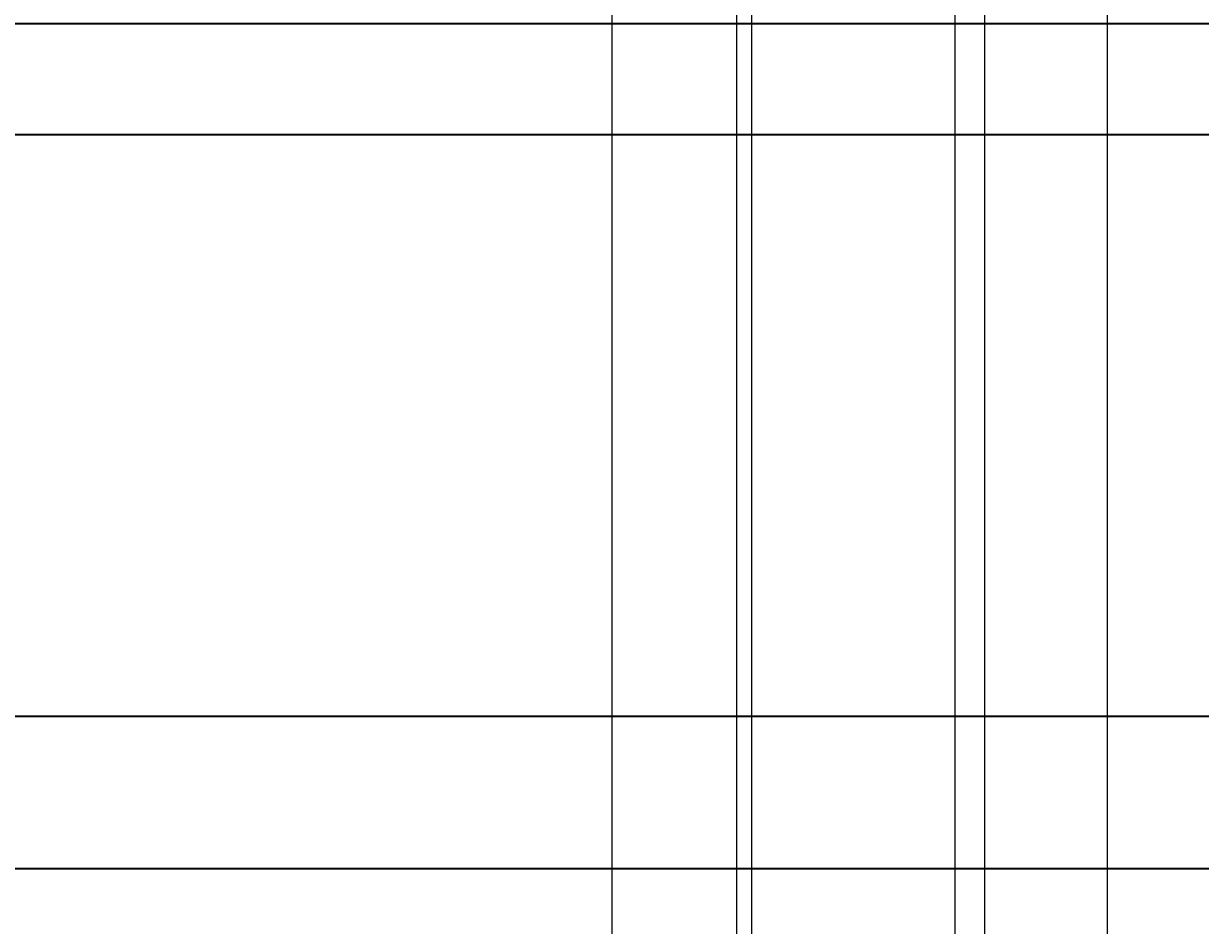
# Model space of a CAD drawing. Units: inches. Extents: x -6 to 289, y -8 to 323.
# Tile 89 of 107: x 150 to 173, y 276 to 294. Entities that reach past the tile are written whole.
import ezdxf

# ---------------------------------------------------------------- set-up
doc = ezdxf.new("R2010")
doc.units = ezdxf.units.IN
doc.header["$MEASUREMENT"] = 0
doc.layers.add('A-ANNO-DIMS', color=2, linetype='Continuous', lineweight=18)
doc.layers.add('A-ELEV', color=7, linetype='Continuous', lineweight=35)
doc.styles.get("Standard").update_dxf_attribs({"font": 'arial.ttf'})
doc.dimstyles.get("Standard").update_dxf_attribs({"dimtxt": 0.18, "dimasz": 0.18, "dimexe": 0.18, "dimexo": 0.0625, "dimgap": 0.09, "dimtad": 0, "dimtih": 1, "dimtoh": 1, "dimdec": 4, "dimzin": 0, "dimdsep": 46, "dimtxsty": 'Standard', "dimcen": 0.09, "dimadec": 0, "dimazin": 0, "dimtfac": 1, "dimtdec": 4, "dimtofl": 0, "dimtmove": 0, "dimatfit": 3, "dimfxl": 1, "dimtolj": 1, "dimtzin": 0, "dimarcsym": 0})

# ---------------------------------------------------------------- blocks, each defined once
blk = doc.blocks.new('*D11')
at = {"layer": 'A-ANNO-DIMS', "color": 0, "lineweight": -2, "transparency": 16777216}
for p, q in [((126.883, 226.717), (126.883, 322.969)), ((168.883, 226.717), (168.883, 322.969)), ((127.063, 322.789), (147.662, 322.789)), ((168.703, 322.789), (148.105, 322.789))]:
    blk.add_line(p, q, dxfattribs=at)
at = {"layer": 'A-ANNO-DIMS', "color": 0, "transparency": 16777216}
for points in [[(127.063, 322.819), (127.063, 322.759), (126.883, 322.789)], [(168.703, 322.819), (168.703, 322.759), (168.883, 322.789)]]:
    blk.add_solid(points, dxfattribs=at)
at = {"layer": 'Defpoints', "color": 0, "transparency": 16777216}
for p in [(168.883, 322.789), (126.883, 226.654), (168.883, 226.654)]:
    blk.add_point(p, dxfattribs=at)
at = {"layer": 'A-ANNO-DIMS', "color": 0, "transparency": 16777216, "insert": (147.883, 322.789), "char_height": 0.18, "attachment_point": 5}
blk.add_mtext('\\A1;42', dxfattribs=at)
blk = doc.blocks.new('*D12')
at = {"layer": 'A-ANNO-DIMS', "color": 0, "lineweight": -2, "transparency": 16777216}
for p, q in [((168.883, 226.717), (168.883, 322.969)), ((188.292, 226.951), (188.292, 322.969)), ((169.063, 322.789), (178.22, 322.789)), ((188.112, 322.789), (178.955, 322.789))]:
    blk.add_line(p, q, dxfattribs=at)
at = {"layer": 'A-ANNO-DIMS', "color": 0, "transparency": 16777216}
for points in [[(169.063, 322.819), (169.063, 322.759), (168.883, 322.789)], [(188.112, 322.819), (188.112, 322.759), (188.292, 322.789)]]:
    blk.add_solid(points, dxfattribs=at)
at = {"layer": 'Defpoints', "color": 0, "transparency": 16777216}
for p in [(188.292, 322.789), (188.292, 226.889), (168.883, 226.654)]:
    blk.add_point(p, dxfattribs=at)
at = {"layer": 'A-ANNO-DIMS', "color": 0, "transparency": 16777216, "insert": (178.588, 322.789), "char_height": 0.18, "attachment_point": 5}
blk.add_mtext('\\A1;19.41', dxfattribs=at)
blk = doc.blocks.new('*D27')
at = {"layer": 'A-ANNO-DIMS', "color": 0, "lineweight": -2, "transparency": 16777216}
for p, q in [((19.226, 307.289), (288.653, 307.289)), ((288.473, 307.109), (288.473, 277.471)), ((288.473, 247.469), (288.473, 277.107)), ((247.226, 247.289), (288.653, 247.289))]:
    blk.add_line(p, q, dxfattribs=at)
at = {"layer": 'A-ANNO-DIMS', "color": 0, "transparency": 16777216}
for points in [[(288.443, 307.109), (288.503, 307.109), (288.473, 307.289)], [(288.443, 247.469), (288.503, 247.469), (288.473, 247.289)]]:
    blk.add_solid(points, dxfattribs=at)
at = {"layer": 'Defpoints', "color": 0, "transparency": 16777216}
for p in [(19.164, 307.289), (288.473, 307.289), (247.164, 247.289)]:
    blk.add_point(p, dxfattribs=at)
at = {"layer": 'A-ANNO-DIMS', "color": 0, "transparency": 16777216, "insert": (288.473, 277.289), "char_height": 0.18, "attachment_point": 5}
blk.add_mtext('\\A1;60', dxfattribs=at)
blk = doc.blocks.new('*D76')
at = {"layer": 'A-ANNO-DIMS', "color": 0, "lineweight": -2, "transparency": 16777216}
for p, q in [((142.296, 51.148), (142.296, 322.969)), ((164.296, 51.148), (164.296, 322.969)), ((142.476, 322.789), (153.076, 322.789)), ((164.116, 322.789), (153.516, 322.789))]:
    blk.add_line(p, q, dxfattribs=at)
at = {"layer": 'A-ANNO-DIMS', "color": 0, "transparency": 16777216}
for points in [[(142.476, 322.819), (142.476, 322.759), (142.296, 322.789)], [(164.116, 322.819), (164.116, 322.759), (164.296, 322.789)]]:
    blk.add_solid(points, dxfattribs=at)
at = {"layer": 'Defpoints', "color": 0, "transparency": 16777216}
for p in [(164.296, 322.789), (142.296, 51.085), (164.296, 51.085)]:
    blk.add_point(p, dxfattribs=at)
at = {"layer": 'A-ANNO-DIMS', "color": 0, "transparency": 16777216, "insert": (153.296, 322.789), "char_height": 0.18, "attachment_point": 5}
blk.add_mtext('\\A1;22', dxfattribs=at)
blk = doc.blocks.new('*D77')
at = {"layer": 'A-ANNO-DIMS', "color": 0, "lineweight": -2, "transparency": 16777216}
for p, q in [((164.296, 51.148), (164.296, 322.969)), ((168.296, 51.148), (168.296, 322.969)), ((164.476, 322.789), (166.144, 322.789)), ((168.116, 322.789), (166.448, 322.789))]:
    blk.add_line(p, q, dxfattribs=at)
at = {"layer": 'A-ANNO-DIMS', "color": 0, "transparency": 16777216}
for points in [[(164.476, 322.819), (164.476, 322.759), (164.296, 322.789)], [(168.116, 322.819), (168.116, 322.759), (168.296, 322.789)]]:
    blk.add_solid(points, dxfattribs=at)
at = {"layer": 'Defpoints', "color": 0, "transparency": 16777216}
for p in [(168.296, 322.789), (164.296, 51.085), (168.296, 51.085)]:
    blk.add_point(p, dxfattribs=at)
at = {"layer": 'A-ANNO-DIMS', "color": 0, "transparency": 16777216, "insert": (166.296, 322.789), "char_height": 0.18, "attachment_point": 5}
blk.add_mtext('\\A1;4', dxfattribs=at)
blk = doc.blocks.new('*D78')
at = {"layer": 'A-ANNO-DIMS', "color": 0, "lineweight": -2, "transparency": 16777216}
for p, q in [((168.296, 51.148), (168.296, 322.969)), ((171.296, 51.148), (171.296, 322.969)), ((168.476, 322.789), (169.647, 322.789)), ((171.116, 322.789), (169.945, 322.789))]:
    blk.add_line(p, q, dxfattribs=at)
at = {"layer": 'A-ANNO-DIMS', "color": 0, "transparency": 16777216}
for points in [[(168.476, 322.819), (168.476, 322.759), (168.296, 322.789)], [(171.116, 322.819), (171.116, 322.759), (171.296, 322.789)]]:
    blk.add_solid(points, dxfattribs=at)
at = {"layer": 'Defpoints', "color": 0, "transparency": 16777216}
for p in [(171.296, 322.789), (168.296, 51.085), (171.296, 51.085)]:
    blk.add_point(p, dxfattribs=at)
at = {"layer": 'A-ANNO-DIMS', "color": 0, "transparency": 16777216, "insert": (169.796, 322.789), "char_height": 0.18, "attachment_point": 5}
blk.add_mtext('\\A1;3', dxfattribs=at)
blk = doc.blocks.new('*D79')
at = {"layer": 'A-ANNO-DIMS', "color": 0, "lineweight": -2, "transparency": 16777216}
for p, q in [((171.296, 118.033), (171.296, 322.969)), ((188.292, 116.842), (188.292, 322.969)), ((171.476, 322.789), (179.339, 322.789)), ((188.112, 322.789), (180.249, 322.789))]:
    blk.add_line(p, q, dxfattribs=at)
at = {"layer": 'A-ANNO-DIMS', "color": 0, "transparency": 16777216}
for points in [[(171.476, 322.819), (171.476, 322.759), (171.296, 322.789)], [(188.112, 322.819), (188.112, 322.759), (188.292, 322.789)]]:
    blk.add_solid(points, dxfattribs=at)
at = {"layer": 'Defpoints', "color": 0, "transparency": 16777216}
for p in [(188.292, 322.789), (171.296, 117.971), (188.292, 116.779)]:
    blk.add_point(p, dxfattribs=at)
at = {"layer": 'A-ANNO-DIMS', "color": 0, "transparency": 16777216, "insert": (179.794, 322.789), "char_height": 0.18, "attachment_point": 5}
blk.add_mtext('\\A1;16.996', dxfattribs=at)
blk = doc.blocks.new('*D94')
at = {"layer": 'A-ANNO-DIMS', "color": 0, "lineweight": -2, "transparency": 16777216}
for p, q in [((118.164, 159.411), (118.164, 322.969)), ((161.552, 159.411), (161.552, 322.969)), ((118.344, 322.789), (139.46, 322.789)), ((161.372, 322.789), (140.256, 322.789))]:
    blk.add_line(p, q, dxfattribs=at)
at = {"layer": 'A-ANNO-DIMS', "color": 0, "transparency": 16777216}
for points in [[(118.344, 322.819), (118.344, 322.759), (118.164, 322.789)], [(161.372, 322.819), (161.372, 322.759), (161.552, 322.789)]]:
    blk.add_solid(points, dxfattribs=at)
at = {"layer": 'Defpoints', "color": 0, "transparency": 16777216}
for p in [(161.552, 322.789), (118.164, 159.348), (161.552, 159.348)]:
    blk.add_point(p, dxfattribs=at)
at = {"layer": 'A-ANNO-DIMS', "color": 0, "transparency": 16777216, "insert": (139.858, 322.789), "char_height": 0.18, "attachment_point": 5}
blk.add_mtext('\\A1;43.39', dxfattribs=at)
blk = doc.blocks.new('*D95')
at = {"layer": 'A-ANNO-DIMS', "color": 0, "lineweight": -2, "transparency": 16777216}
for p, q in [((161.552, 159.411), (161.552, 322.969)), ((164.004, 159.411), (164.004, 322.969)), ((161.732, 322.789), (162.452, 322.789)), ((163.824, 322.789), (163.104, 322.789))]:
    blk.add_line(p, q, dxfattribs=at)
at = {"layer": 'A-ANNO-DIMS', "color": 0, "transparency": 16777216}
for points in [[(161.732, 322.819), (161.732, 322.759), (161.552, 322.789)], [(163.824, 322.819), (163.824, 322.759), (164.004, 322.789)]]:
    blk.add_solid(points, dxfattribs=at)
at = {"layer": 'Defpoints', "color": 0, "transparency": 16777216}
for p in [(164.004, 322.789), (161.552, 159.348), (164.004, 159.348)]:
    blk.add_point(p, dxfattribs=at)
at = {"layer": 'A-ANNO-DIMS', "color": 0, "transparency": 16777216, "insert": (162.778, 322.789), "char_height": 0.18, "attachment_point": 5}
blk.add_mtext('\\A1;2.45', dxfattribs=at)
blk = doc.blocks.new('*D96')
at = {"layer": 'A-ANNO-DIMS', "color": 0, "lineweight": -2, "transparency": 16777216}
for p, q in [((164.004, 159.411), (164.004, 322.969)), ((200.616, 159.411), (200.616, 322.969)), ((164.184, 322.789), (181.934, 322.789)), ((200.436, 322.789), (182.686, 322.789))]:
    blk.add_line(p, q, dxfattribs=at)
at = {"layer": 'A-ANNO-DIMS', "color": 0, "transparency": 16777216}
for points in [[(164.184, 322.819), (164.184, 322.759), (164.004, 322.789)], [(200.436, 322.819), (200.436, 322.759), (200.616, 322.789)]]:
    blk.add_solid(points, dxfattribs=at)
at = {"layer": 'Defpoints', "color": 0, "transparency": 16777216}
for p in [(200.616, 322.789), (164.004, 159.348), (200.616, 159.348)]:
    blk.add_point(p, dxfattribs=at)
at = {"layer": 'A-ANNO-DIMS', "color": 0, "transparency": 16777216, "insert": (182.31, 322.789), "char_height": 0.18, "attachment_point": 5}
blk.add_mtext('\\A1;36.61', dxfattribs=at)
blk = doc.blocks.new('*D107')
at = {"layer": 'A-ANNO-DIMS', "color": 0, "lineweight": -2, "transparency": 16777216}
for p, q in [((118.164, 293.728), (118.164, 322.969)), ((186.984, 291.541), (186.984, 322.969)), ((118.344, 322.789), (152.18, 322.789)), ((186.804, 322.789), (152.967, 322.789))]:
    blk.add_line(p, q, dxfattribs=at)
at = {"layer": 'A-ANNO-DIMS', "color": 0, "transparency": 16777216}
for points in [[(118.344, 322.819), (118.344, 322.759), (118.164, 322.789)], [(186.804, 322.819), (186.804, 322.759), (186.984, 322.789)]]:
    blk.add_solid(points, dxfattribs=at)
at = {"layer": 'Defpoints', "color": 0, "transparency": 16777216}
for p in [(186.984, 322.789), (118.164, 293.666), (186.984, 291.478)]:
    blk.add_point(p, dxfattribs=at)
at = {"layer": 'A-ANNO-DIMS', "color": 0, "transparency": 16777216, "insert": (152.574, 322.789), "char_height": 0.18, "attachment_point": 5}
blk.add_mtext('\\A1;68.82', dxfattribs=at)

msp = doc.modelspace()

# ---------------------------------------------------------------- linework, layer by layer
at = {"layer": 'A-ELEV'}
for points in [[(115.1638, 307.2888), (115.1638, 277.0427), (259.1638, 277.0427), (259.1638, 259.2888)], [(118.1638, 307.2888), (118.1638, 280.0427), (262.1638, 280.0427), (262.1638, 259.2888)], [(255.8036, 291.4781), (118.1638, 291.4781), (118.1638, 293.6657), (255.8036, 293.6657)]]:
    msp.add_lwpolyline(points, dxfattribs=at)

# ---------------------------------------------------------------- dimensions: what is measured, and where the dimension line sits
at = {"layer": 'A-ANNO-DIMS'}
for base, p1, p2, override, picture, middle in [((161.5522, 322.7888), (118.1638, 159.3484), (161.5522, 159.3484), {"dimdec": 2, "dimlfac": 1, "dimrnd": 0, "dimzin": 0, "dimdsep": 46, "dimlunit": 2}, '*D94', (139.858, 322.7888)), ((186.9837, 322.7888), (118.1638, 293.6657), (186.9837, 291.4781), {"dimdec": 2, "dimlfac": 1, "dimrnd": 0, "dimzin": 0, "dimdsep": 46, "dimlunit": 2}, '*D107', (152.5737, 322.7888)), ((168.8835, 322.7888), (126.8835, 226.654), (168.8835, 226.654), {"dimdec": 0, "dimlfac": 1, "dimrnd": 0, "dimzin": 0, "dimdsep": 46, "dimlunit": 2}, '*D11', (147.8835, 322.7888)), ((164.296, 322.7888), (142.296, 51.0851), (164.296, 51.0851), {"dimdec": 0, "dimlfac": 1, "dimrnd": 0, "dimzin": 0, "dimdsep": 46, "dimlunit": 2}, '*D76', (153.296, 322.7888)), ((164.0039, 322.7888), (161.5522, 159.3484), (164.0039, 159.3484), {"dimdec": 2, "dimlfac": 1, "dimrnd": 0, "dimzin": 0, "dimdsep": 46, "dimlunit": 2}, '*D95', (162.7781, 322.7888)), ((200.6162, 322.7888), (164.0039, 159.3484), (200.6162, 159.3484), {"dimdec": 2, "dimlfac": 1, "dimrnd": 0, "dimzin": 0, "dimdsep": 46, "dimlunit": 2}, '*D96', (182.3101, 322.7888)), ((168.296, 322.7888), (164.296, 51.0851), (168.296, 51.0851), {"dimdec": 0, "dimlfac": 1, "dimrnd": 0, "dimzin": 0, "dimdsep": 46, "dimlunit": 2}, '*D77', (166.296, 322.7888)), ((171.296, 322.7888), (168.296, 51.0851), (171.296, 51.0851), {"dimdec": 0, "dimlfac": 1, "dimrnd": 0, "dimzin": 0, "dimdsep": 46, "dimlunit": 2}, '*D78', (169.796, 322.7888)), ((188.2918, 322.7888), (168.8835, 226.654), (188.2918, 226.8887), {"dimdec": 2, "dimlfac": 1, "dimrnd": 0, "dimzin": 0, "dimdsep": 46, "dimlunit": 2}, '*D12', (178.5876, 322.7888)), ((188.2918, 322.7888), (171.296, 117.9706), (188.2918, 116.7795), {"dimdec": 3, "dimlfac": 1, "dimrnd": 0, "dimzin": 0, "dimdsep": 46, "dimlunit": 2}, '*D79', (179.7939, 322.7888))]:
    dim = msp.add_linear_dim(base=base, p1=p1, p2=p2, dimstyle='Standard', override=override, dxfattribs=at)
    dim.commit()
    dim.dimension.update_dxf_attribs({"geometry": picture, "text_midpoint": middle})
dim = msp.add_linear_dim(base=(288.4733, 307.2888), p1=(247.1638, 247.2888), p2=(19.1638, 307.2888), angle=90, dimstyle='Standard', override={"dimdec": 0, "dimlfac": 1, "dimrnd": 0, "dimzin": 0, "dimdsep": 46, "dimlunit": 2}, dxfattribs=at)
dim.commit()
dim.dimension.update_dxf_attribs({"geometry": '*D27', "text_midpoint": (288.4733, 277.2888)})

doc.saveas('drawing.dxf')
